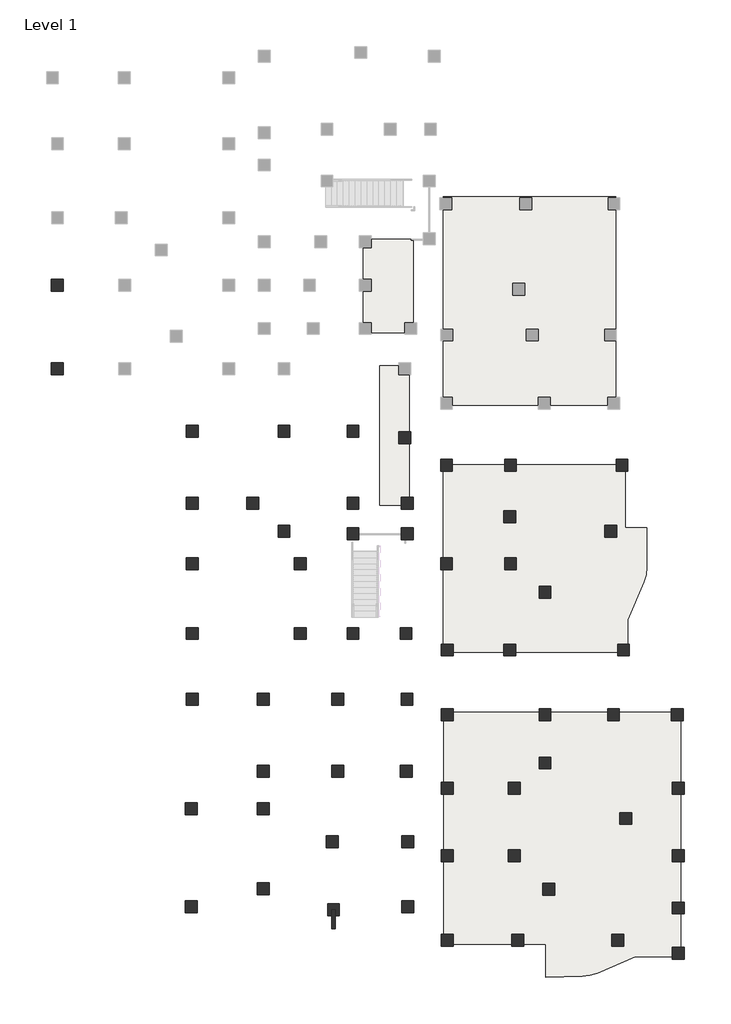
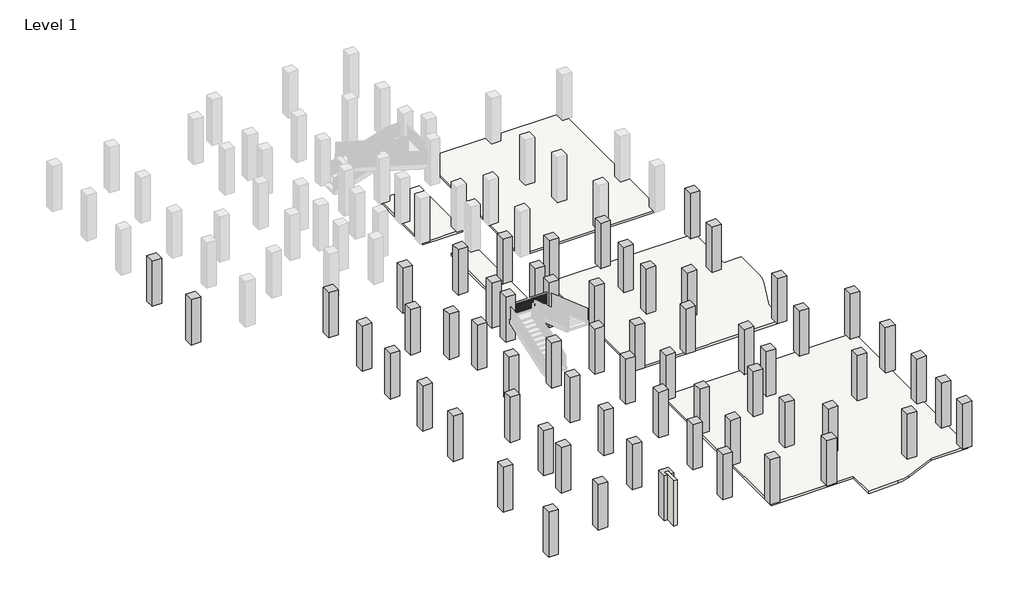
# One storey, part 1 of 6: 63 columns, 6 slabs, 1 wall.
"""IFC4 building model written with IfcOpenShell, lengths in millimetres."""

from ifc_helpers import new_model, si_unit, point, frame, frame_2d, origin, origin_with_axes, place, context, project, spatial, polyline, circle_curve, trimmed, segment, composite_curve, outline, extrude, faceted_brep, element, save

model = new_model("IFC4")

# Units and contexts
model_context = context("Model", 3, world=origin())
ifc_project = project(units=[si_unit("LENGTHUNIT", "METRE", prefix="MILLI")], contexts=[model_context])

# Site, building, storey
site = spatial("IfcSite", under=ifc_project)
building = spatial("IfcBuilding", under=site)
storey = spatial("IfcBuildingStorey", under=building, Name="Level 1", Elevation=0.0)

# Columns
placement = place(None, origin())
element("IfcColumn", 1, ObjectType="Rectangular Column : 24\" x 24\"", at=placement, inside=storey, context=model_context, shape_type="SweptSolid", body=[
    extrude(outline(polyline([(-4542.8891351, -24693.9416506), (-4542.8891351, -25303.5416506), (-4746.0891351, -25303.5416506), (-4746.0891351, -24998.7416506), (-4949.2891351, -24998.7416506), (-4949.2891351, -25303.5416506), (-5152.4891351, -25303.5416506), (-5152.4891351, -24693.9416506), (-4542.8891351, -24693.9416506)])), origin_with_axes(), (0.0, 0.0, 1.0), 3048.0),
])
element("IfcColumn", 2, ObjectType="Rectangular Column : 24\" x 24\"", at=placement, inside=storey, context=model_context, shape_type="SweptSolid", body=[
    extrude(outline(polyline([(-4321.237215, -17586.4072331), (-4321.237215, -18196.0072331), (-4930.837215, -18196.0072331), (-4930.837215, -17586.4072331), (-4321.237215, -17586.4072331)])), origin_with_axes(), (0.0, 0.0, 1.0), 3048.0),
])
element("IfcColumn", 3, ObjectType="Rectangular Column : 24\" x 24\"", at=placement, inside=storey, context=model_context, shape_type="SweptSolid", body=[
    extrude(outline(polyline([(-4600.0391351, -21207.7916506), (-4600.0391351, -21817.3916506), (-5209.6391351, -21817.3916506), (-5209.6391351, -21207.7916506), (-4600.0391351, -21207.7916506)])), origin_with_axes(), (0.0, 0.0, 1.0), 3048.0),
])
element("IfcColumn", 4, ObjectType="Rectangular Column : 24\" x 24\"", at=placement, inside=storey, context=model_context, shape_type="SweptSolid", body=[
    extrude(outline(polyline([(-11810.6574308, -13883.8238356), (-11810.6574308, -14493.4238356), (-12420.2574308, -14493.4238356), (-12420.2574308, -13883.8238356), (-11810.6574308, -13883.8238356)])), origin_with_axes(), (0.0, 0.0, 1.0), 3048.0),
])
element("IfcColumn", 5, ObjectType="Rectangular Column : 24\" x 24\"", at=placement, inside=storey, context=model_context, shape_type="SweptSolid", body=[
    extrude(outline(polyline([(-8149.0858024, -13883.8238356), (-8149.0858024, -14493.4238356), (-8758.6858024, -14493.4238356), (-8758.6858024, -13883.8238356), (-8149.0858024, -13883.8238356)])), origin_with_axes(), (0.0, 0.0, 1.0), 3048.0),
])
element("IfcColumn", 6, ObjectType="Rectangular Column : 24\" x 24\"", at=placement, inside=storey, context=model_context, shape_type="SweptSolid", body=[
    extrude(outline(polyline([(-4321.237215, -13883.8238356), (-4321.237215, -14493.4238356), (-4930.837215, -14493.4238356), (-4930.837215, -13883.8238356), (-4321.237215, -13883.8238356)])), origin_with_axes(), (0.0, 0.0, 1.0), 3048.0),
])
element("IfcColumn", 7, ObjectType="Rectangular Column : 24\" x 24\"", at=placement, inside=storey, context=model_context, shape_type="SweptSolid", body=[
    extrude(outline(polyline([(-766.6425319, -13883.8238356), (-766.6425319, -14493.4238356), (-1376.2425319, -14493.4238356), (-1376.2425319, -13883.8238356), (-766.6425319, -13883.8238356)])), origin_with_axes(), (0.0, 0.0, 1.0), 3048.0),
])
element("IfcColumn", 8, ObjectType="Rectangular Column : 24\" x 24\"", at=placement, inside=storey, context=model_context, shape_type="SweptSolid", body=[
    extrude(outline(polyline([(-794.2108128, -17586.4072331), (-794.2108128, -18196.0072331), (-1403.8108128, -18196.0072331), (-1403.8108128, -17586.4072331), (-794.2108128, -17586.4072331)])), origin_with_axes(), (0.0, 0.0, 1.0), 3048.0),
])
element("IfcColumn", 9, ObjectType="Rectangular Column : 24\" x 24\"", at=placement, inside=storey, context=model_context, shape_type="SweptSolid", body=[
    extrude(outline(polyline([(-732.8891351, -21207.7916506), (-732.8891351, -21817.3916506), (-1342.4891351, -21817.3916506), (-1342.4891351, -21207.7916506), (-732.8891351, -21207.7916506)])), origin_with_axes(), (0.0, 0.0, 1.0), 3048.0),
])
element("IfcColumn", 10, ObjectType="Rectangular Column : 24\" x 24\"", at=placement, inside=storey, context=model_context, shape_type="SweptSolid", body=[
    extrude(outline(polyline([(-732.8891351, -24541.5416506), (-732.8891351, -25151.1416506), (-1342.4891351, -25151.1416506), (-1342.4891351, -24541.5416506), (-732.8891351, -24541.5416506)])), origin_with_axes(), (0.0, 0.0, 1.0), 3048.0),
])
element("IfcColumn", 11, ObjectType="Rectangular Column : 24\" x 24\"", at=placement, inside=storey, context=model_context, shape_type="SweptSolid", body=[
    extrude(outline(polyline([(-11858.0891351, -24541.5416506), (-11858.0891351, -25151.1416506), (-12467.6891351, -25151.1416506), (-12467.6891351, -24541.5416506), (-11858.0891351, -24541.5416506)])), origin_with_axes(), (0.0, 0.0, 1.0), 3048.0),
])
element("IfcColumn", 12, ObjectType="Rectangular Column : 24\" x 24\"", at=placement, inside=storey, context=model_context, shape_type="SweptSolid", body=[
    extrude(outline(polyline([(-11858.0891351, -19512.3416506), (-11858.0891351, -20121.9416506), (-12467.6891351, -20121.9416506), (-12467.6891351, -19512.3416506), (-11858.0891351, -19512.3416506)])), origin_with_axes(), (0.0, 0.0, 1.0), 3048.0),
])
element("IfcColumn", 13, ObjectType="Rectangular Column : 24\" x 24\"", at=placement, inside=storey, context=model_context, shape_type="SweptSolid", body=[
    extrude(outline(polyline([(-8149.0858024, -17586.4072331), (-8149.0858024, -18196.0072331), (-8758.6858024, -18196.0072331), (-8758.6858024, -17586.4072331), (-8149.0858024, -17586.4072331)])), origin_with_axes(), (0.0, 0.0, 1.0), 3048.0),
])
element("IfcColumn", 14, ObjectType="Rectangular Column : 24\" x 24\"", at=placement, inside=storey, context=model_context, shape_type="SweptSolid", body=[
    extrude(outline(polyline([(-8149.0858024, -19512.3416506), (-8149.0858024, -20121.9416506), (-8758.6858024, -20121.9416506), (-8758.6858024, -19512.3416506), (-8149.0858024, -19512.3416506)])), origin_with_axes(), (0.0, 0.0, 1.0), 3048.0),
])
element("IfcColumn", 15, ObjectType="Rectangular Column : 24\" x 24\"", at=placement, inside=storey, context=model_context, shape_type="SweptSolid", body=[
    extrude(outline(polyline([(-8149.0858024, -23627.1416506), (-8149.0858024, -24236.7416506), (-8758.6858024, -24236.7416506), (-8758.6858024, -23627.1416506), (-8149.0858024, -23627.1416506)])), origin_with_axes(), (0.0, 0.0, 1.0), 3048.0),
])
element("IfcColumn", 16, ObjectType="Rectangular Column : 24\" x 24\"", at=placement, inside=storey, context=model_context, shape_type="SweptSolid", body=[
    extrude(outline(polyline([(1308.8550323, -26276.0205306), (1308.8550323, -26885.6205306), (699.2550323, -26885.6205306), (699.2550323, -26276.0205306), (1308.8550323, -26276.0205306)])), origin_with_axes(), (0.0, 0.0, 1.0), 3048.0),
])
element("IfcColumn", 17, ObjectType="Rectangular Column : 24\" x 24\"", at=placement, inside=storey, context=model_context, shape_type="SweptSolid", body=[
    extrude(outline(polyline([(4934.0839763, -26276.0205306), (4934.0839763, -26885.6205306), (4324.4839763, -26885.6205306), (4324.4839763, -26276.0205306), (4934.0839763, -26276.0205306)])), origin_with_axes(), (0.0, 0.0, 1.0), 3048.0),
])
element("IfcColumn", 18, ObjectType="Rectangular Column : 24\" x 24\"", at=placement, inside=storey, context=model_context, shape_type="SweptSolid", body=[
    extrude(outline(polyline([(1308.8550323, -21920.2321416), (1308.8550323, -22529.8321416), (699.2550323, -22529.8321416), (699.2550323, -21920.2321416), (1308.8550323, -21920.2321416)])), origin_with_axes(), (0.0, 0.0, 1.0), 3048.0),
])
element("IfcColumn", 19, ObjectType="Rectangular Column : 24\" x 24\"", at=placement, inside=storey, context=model_context, shape_type="SweptSolid", body=[
    extrude(outline(polyline([(1308.8550323, -18453.3485113), (1308.8550323, -19062.9485113), (699.2550323, -19062.9485113), (699.2550323, -18453.3485113), (1308.8550323, -18453.3485113)])), origin_with_axes(), (0.0, 0.0, 1.0), 3048.0),
])
element("IfcColumn", 20, ObjectType="Rectangular Column : 24\" x 24\"", at=placement, inside=storey, context=model_context, shape_type="SweptSolid", body=[
    extrude(outline(polyline([(1308.8550323, -14677.1022473), (1308.8550323, -15286.7022473), (699.2550323, -15286.7022473), (699.2550323, -14677.1022473), (1308.8550323, -14677.1022473)])), origin_with_axes(), (0.0, 0.0, 1.0), 3048.0),
])
element("IfcColumn", 21, ObjectType="Rectangular Column : 24\" x 24\"", at=placement, inside=storey, context=model_context, shape_type="SweptSolid", body=[
    extrude(outline(polyline([(1308.8550323, -11343.8334596), (1308.8550323, -11953.4334596), (699.2550323, -11953.4334596), (699.2550323, -11343.8334596), (1308.8550323, -11343.8334596)])), origin_with_axes(), (0.0, 0.0, 1.0), 3048.0),
])
element("IfcColumn", 22, ObjectType="Rectangular Column : 24\" x 24\"", at=placement, inside=storey, context=model_context, shape_type="SweptSolid", body=[
    extrude(outline(polyline([(6333.7118156, -14677.1022473), (6333.7118156, -15286.7022473), (5724.1118156, -15286.7022473), (5724.1118156, -14677.1022473), (6333.7118156, -14677.1022473)])), origin_with_axes(), (0.0, 0.0, 1.0), 3048.0),
])
element("IfcColumn", 23, ObjectType="Rectangular Column : 24\" x 24\"", at=placement, inside=storey, context=model_context, shape_type="SweptSolid", body=[
    extrude(outline(polyline([(9855.6561951, -14677.1022473), (9855.6561951, -15286.7022473), (9246.0561951, -15286.7022473), (9246.0561951, -14677.1022473), (9855.6561951, -14677.1022473)])), origin_with_axes(), (0.0, 0.0, 1.0), 3048.0),
])
element("IfcColumn", 24, ObjectType="Rectangular Column : 24\" x 24\"", at=placement, inside=storey, context=model_context, shape_type="SweptSolid", body=[
    extrude(outline(polyline([(13126.0331188, -14677.1022473), (13126.0331188, -15286.7022473), (12516.4331188, -15286.7022473), (12516.4331188, -14677.1022473), (13126.0331188, -14677.1022473)])), origin_with_axes(), (0.0, 0.0, 1.0), 3048.0),
])
element("IfcColumn", 25, ObjectType="Rectangular Column : 24\" x 24\"", at=placement, inside=storey, context=model_context, shape_type="SweptSolid", body=[
    extrude(outline(polyline([(13188.9249828, -18453.3485113), (13188.9249828, -19062.9485113), (12579.3249828, -19062.9485113), (12579.3249828, -18453.3485113), (13188.9249828, -18453.3485113)])), origin_with_axes(), (0.0, 0.0, 1.0), 3048.0),
])
element("IfcColumn", 26, ObjectType="Rectangular Column : 24\" x 24\"", at=placement, inside=storey, context=model_context, shape_type="SweptSolid", body=[
    extrude(outline(polyline([(13188.9249828, -21920.2321416), (13188.9249828, -22529.8321416), (12579.3249828, -22529.8321416), (12579.3249828, -21920.2321416), (13188.9249828, -21920.2321416)])), origin_with_axes(), (0.0, 0.0, 1.0), 3048.0),
])
element("IfcColumn", 27, ObjectType="Rectangular Column : 24\" x 24\"", at=placement, inside=storey, context=model_context, shape_type="SweptSolid", body=[
    extrude(outline(polyline([(13188.9249828, -24614.0167464), (13188.9249828, -25223.6167464), (12579.3249828, -25223.6167464), (12579.3249828, -24614.0167464), (13188.9249828, -24614.0167464)])), origin_with_axes(), (0.0, 0.0, 1.0), 3048.0),
])
element("IfcColumn", 28, ObjectType="Rectangular Column : 24\" x 24\"", at=placement, inside=storey, context=model_context, shape_type="SweptSolid", body=[
    extrude(outline(polyline([(13188.9249828, -26941.0157114), (13188.9249828, -27550.6157114), (12579.3249828, -27550.6157114), (12579.3249828, -26941.0157114), (13188.9249828, -26941.0157114)])), origin_with_axes(), (0.0, 0.0, 1.0), 3048.0),
])
element("IfcColumn", 29, ObjectType="Rectangular Column : 24\" x 24\"", at=placement, inside=storey, context=model_context, shape_type="SweptSolid", body=[
    extrude(outline(polyline([(6531.1948888, -23643.0476028), (6531.1948888, -24252.6476028), (5921.5948888, -24252.6476028), (5921.5948888, -23643.0476028), (6531.1948888, -23643.0476028)])), origin_with_axes(), (0.0, 0.0, 1.0), 3048.0),
])
element("IfcColumn", 30, ObjectType="Rectangular Column : 24\" x 24\"", at=placement, inside=storey, context=model_context, shape_type="SweptSolid", body=[
    extrude(outline(polyline([(6330.6701053, -17153.3364275), (6330.6701053, -17762.9364275), (5721.0701053, -17762.9364275), (5721.0701053, -17153.3364275), (6330.6701053, -17153.3364275)])), origin_with_axes(), (0.0, 0.0, 1.0), 3048.0),
])
element("IfcColumn", 31, ObjectType="Rectangular Column : 24\" x 24\"", at=placement, inside=storey, context=model_context, shape_type="SweptSolid", body=[
    extrude(outline(polyline([(4744.701363, -18453.3485113), (4744.701363, -19062.9485113), (4135.101363, -19062.9485113), (4135.101363, -18453.3485113), (4744.701363, -18453.3485113)])), origin_with_axes(), (0.0, 0.0, 1.0), 3048.0),
])
element("IfcColumn", 32, ObjectType="Rectangular Column : 24\" x 24\"", at=placement, inside=storey, context=model_context, shape_type="SweptSolid", body=[
    extrude(outline(polyline([(4744.701363, -21920.2321416), (4744.701363, -22529.8321416), (4135.101363, -22529.8321416), (4135.101363, -21920.2321416), (4744.701363, -21920.2321416)])), origin_with_axes(), (0.0, 0.0, 1.0), 3048.0),
])
element("IfcColumn", 33, ObjectType="Rectangular Column : 24\" x 24\"", at=placement, inside=storey, context=model_context, shape_type="SweptSolid", body=[
    extrude(outline(polyline([(10492.7602331, -20012.0333502), (10492.7602331, -20621.6333502), (9883.1602331, -20621.6333502), (9883.1602331, -20012.0333502), (10492.7602331, -20012.0333502)])), origin_with_axes(), (0.0, 0.0, 1.0), 3048.0),
])
element("IfcColumn", 34, ObjectType="Rectangular Column : 24\" x 24\"", at=placement, inside=storey, context=model_context, shape_type="SweptSolid", body=[
    extrude(outline(polyline([(10072.0128709, -26276.0205306), (10072.0128709, -26885.6205306), (9462.4128709, -26885.6205306), (9462.4128709, -26276.0205306), (10072.0128709, -26276.0205306)])), origin_with_axes(), (0.0, 0.0, 1.0), 3048.0),
])
element("IfcColumn", 35, ObjectType="Rectangular Column : 24\" x 24\"", at=placement, inside=storey, context=model_context, shape_type="SweptSolid", body=[
    extrude(outline(polyline([(4518.3886201, -11343.8334596), (4518.3886201, -11953.4334596), (3908.7886201, -11953.4334596), (3908.7886201, -11343.8334596), (4518.3886201, -11343.8334596)])), origin_with_axes(), (0.0, 0.0, 1.0), 3048.0),
])
element("IfcColumn", 36, ObjectType="Rectangular Column : 24\" x 24\"", at=placement, inside=storey, context=model_context, shape_type="SweptSolid", body=[
    extrude(outline(polyline([(10367.3319646, -11343.8334596), (10367.3319646, -11953.4334596), (9757.7319646, -11953.4334596), (9757.7319646, -11343.8334596), (10367.3319646, -11343.8334596)])), origin_with_axes(), (0.0, 0.0, 1.0), 3048.0),
])
element("IfcColumn", 37, ObjectType="Rectangular Column : 24\" x 24\"", at=placement, inside=storey, context=model_context, shape_type="SweptSolid", body=[
    extrude(outline(polyline([(4560.3165294, -6918.1541185), (4560.3165294, -7527.7541185), (3950.7165294, -7527.7541185), (3950.7165294, -6918.1541185), (4560.3165294, -6918.1541185)])), origin_with_axes(), (0.0, 0.0, 1.0), 3048.0),
])
element("IfcColumn", 38, ObjectType="Rectangular Column : 24\" x 24\"", at=placement, inside=storey, context=model_context, shape_type="SweptSolid", body=[
    extrude(outline(polyline([(1268.975651, -6918.1541185), (1268.975651, -7527.7541185), (659.375651, -7527.7541185), (659.375651, -6918.1541185), (1268.975651, -6918.1541185)])), origin_with_axes(), (0.0, 0.0, 1.0), 3048.0),
])
element("IfcColumn", 39, ObjectType="Rectangular Column : 24\" x 24\"", at=placement, inside=storey, context=model_context, shape_type="SweptSolid", body=[
    extrude(outline(polyline([(1268.975651, -1847.7319933), (1268.975651, -2457.3319933), (659.375651, -2457.3319933), (659.375651, -1847.7319933), (1268.975651, -1847.7319933)])), origin_with_axes(), (0.0, 0.0, 1.0), 3048.0),
])
element("IfcColumn", 40, ObjectType="Rectangular Column : 24\" x 24\"", at=placement, inside=storey, context=model_context, shape_type="SweptSolid", body=[
    extrude(outline(polyline([(4560.3165294, -1847.7319933), (4560.3165294, -2457.3319933), (3950.7165294, -2457.3319933), (3950.7165294, -1847.7319933), (4560.3165294, -1847.7319933)])), origin_with_axes(), (0.0, 0.0, 1.0), 3048.0),
])
element("IfcColumn", 41, ObjectType="Rectangular Column : 24\" x 24\"", at=placement, inside=storey, context=model_context, shape_type="SweptSolid", body=[
    extrude(outline(polyline([(10293.0740996, -1847.7319933), (10293.0740996, -2457.3319933), (9683.4740996, -2457.3319933), (9683.4740996, -1847.7319933), (10293.0740996, -1847.7319933)])), origin_with_axes(), (0.0, 0.0, 1.0), 3048.0),
])
element("IfcColumn", 42, ObjectType="Rectangular Column : 24\" x 24\"", at=placement, inside=storey, context=model_context, shape_type="SweptSolid", body=[
    extrude(outline(polyline([(9706.0833697, -5246.6270738), (9706.0833697, -5856.2270738), (9096.4833697, -5856.2270738), (9096.4833697, -5246.6270738), (9706.0833697, -5246.6270738)])), origin_with_axes(), (0.0, 0.0, 1.0), 3048.0),
])
element("IfcColumn", 43, ObjectType="Rectangular Column : 24\" x 24\"", at=placement, inside=storey, context=model_context, shape_type="SweptSolid", body=[
    extrude(outline(polyline([(6333.7118156, -8377.9582897), (6333.7118156, -8987.5582897), (5724.1118156, -8987.5582897), (5724.1118156, -8377.9582897), (6333.7118156, -8377.9582897)])), origin_with_axes(), (0.0, 0.0, 1.0), 3048.0),
])
element("IfcColumn", 44, ObjectType="Rectangular Column : 24\" x 24\"", at=placement, inside=storey, context=model_context, shape_type="SweptSolid", body=[
    extrude(outline(polyline([(4518.3886201, -4496.4820882), (4518.3886201, -5106.0820882), (3908.7886201, -5106.0820882), (3908.7886201, -4496.4820882), (4518.3886201, -4496.4820882)])), origin_with_axes(), (0.0, 0.0, 1.0), 3048.0),
])
element("IfcColumn", 45, ObjectType="Rectangular Column : 24\" x 24\"", at=placement, inside=storey, context=model_context, shape_type="SweptSolid", body=[
    extrude(outline(polyline([(-3540.2090245, -3808.9159518), (-3540.2090245, -4418.5159518), (-4149.8090245, -4418.5159518), (-4149.8090245, -3808.9159518), (-3540.2090245, -3808.9159518)])), origin_with_axes(), (0.0, 0.0, 1.0), 3048.0),
])
element("IfcColumn", 46, ObjectType="Rectangular Column : 24\" x 24\"", at=placement, inside=storey, context=model_context, shape_type="SweptSolid", body=[
    extrude(outline(polyline([(-3540.2090245, -5366.5238251), (-3540.2090245, -5976.1238251), (-4149.8090245, -5976.1238251), (-4149.8090245, -5366.5238251), (-3540.2090245, -5366.5238251)])), origin_with_axes(), (0.0, 0.0, 1.0), 3048.0),
])
element("IfcColumn", 47, ObjectType="Rectangular Column : 24\" x 24\"", at=placement, inside=storey, context=model_context, shape_type="SweptSolid", body=[
    extrude(outline(polyline([(-742.0285088, -5366.5238251), (-742.0285088, -5976.1238251), (-1351.6285088, -5976.1238251), (-1351.6285088, -5366.5238251), (-742.0285088, -5366.5238251)])), origin_with_axes(), (0.0, 0.0, 1.0), 3048.0),
])
element("IfcColumn", 48, ObjectType="Rectangular Column : 24\" x 24\"", at=placement, inside=storey, context=model_context, shape_type="SweptSolid", body=[
    extrude(outline(polyline([(-811.1636894, -10494.4811097), (-811.1636894, -11104.0811097), (-1420.7636894, -11104.0811097), (-1420.7636894, -10494.4811097), (-811.1636894, -10494.4811097)])), origin_with_axes(), (0.0, 0.0, 1.0), 3048.0),
])
element("IfcColumn", 49, ObjectType="Rectangular Column : 24\" x 24\"", at=placement, inside=storey, context=model_context, shape_type="SweptSolid", body=[
    extrude(outline(polyline([(-3540.2090245, -10494.4811097), (-3540.2090245, -11104.0811097), (-4149.8090245, -11104.0811097), (-4149.8090245, -10494.4811097), (-3540.2090245, -10494.4811097)])), origin_with_axes(), (0.0, 0.0, 1.0), 3048.0),
])
element("IfcColumn", 50, ObjectType="Rectangular Column : 24\" x 24\"", at=placement, inside=storey, context=model_context, shape_type="SweptSolid", body=[
    extrude(outline(polyline([(-6255.1201851, -10494.4811097), (-6255.1201851, -11104.0811097), (-6864.7201851, -11104.0811097), (-6864.7201851, -10494.4811097), (-6255.1201851, -10494.4811097)])), origin_with_axes(), (0.0, 0.0, 1.0), 3048.0),
])
element("IfcColumn", 51, ObjectType="Rectangular Column : 24\" x 24\"", at=placement, inside=storey, context=model_context, shape_type="SweptSolid", body=[
    extrude(outline(polyline([(-11810.6574308, -10494.4811097), (-11810.6574308, -11104.0811097), (-12420.2574308, -11104.0811097), (-12420.2574308, -10494.4811097), (-11810.6574308, -10494.4811097)])), origin_with_axes(), (0.0, 0.0, 1.0), 3048.0),
])
element("IfcColumn", 52, ObjectType="Rectangular Column : 24\" x 24\"", at=placement, inside=storey, context=model_context, shape_type="SweptSolid", body=[
    extrude(outline(polyline([(-6255.1201851, -6918.1541185), (-6255.1201851, -7527.7541185), (-6864.7201851, -7527.7541185), (-6864.7201851, -6918.1541185), (-6255.1201851, -6918.1541185)])), origin_with_axes(), (0.0, 0.0, 1.0), 3048.0),
])
element("IfcColumn", 53, ObjectType="Rectangular Column : 24\" x 24\"", at=placement, inside=storey, context=model_context, shape_type="SweptSolid", body=[
    extrude(outline(polyline([(-11810.6574308, -6918.1541185), (-11810.6574308, -7527.7541185), (-12420.2574308, -7527.7541185), (-12420.2574308, -6918.1541185), (-11810.6574308, -6918.1541185)])), origin_with_axes(), (0.0, 0.0, 1.0), 3048.0),
])
element("IfcColumn", 54, ObjectType="Rectangular Column : 24\" x 24\"", at=placement, inside=storey, context=model_context, shape_type="SweptSolid", body=[
    extrude(outline(polyline([(-7086.8650855, -5246.6270738), (-7086.8650855, -5856.2270738), (-7696.4650855, -5856.2270738), (-7696.4650855, -5246.6270738), (-7086.8650855, -5246.6270738)])), origin_with_axes(), (0.0, 0.0, 1.0), 3048.0),
])
element("IfcColumn", 55, ObjectType="Rectangular Column : 24\" x 24\"", at=placement, inside=storey, context=model_context, shape_type="SweptSolid", body=[
    extrude(outline(polyline([(-8694.9052261, -3808.9159518), (-8694.9052261, -4418.5159518), (-9304.5052261, -4418.5159518), (-9304.5052261, -3808.9159518), (-8694.9052261, -3808.9159518)])), origin_with_axes(), (0.0, 0.0, 1.0), 3048.0),
])
element("IfcColumn", 56, ObjectType="Rectangular Column : 24\" x 24\"", at=placement, inside=storey, context=model_context, shape_type="SweptSolid", body=[
    extrude(outline(polyline([(-11810.6574308, -3808.9159518), (-11810.6574308, -4418.5159518), (-12420.2574308, -4418.5159518), (-12420.2574308, -3808.9159518), (-11810.6574308, -3808.9159518)])), origin_with_axes(), (0.0, 0.0, 1.0), 3048.0),
])
element("IfcColumn", 57, ObjectType="Rectangular Column : 24\" x 24\"", at=placement, inside=storey, context=model_context, shape_type="SweptSolid", body=[
    extrude(outline(polyline([(-11810.6574308, -106.2126672), (-11810.6574308, -715.8126672), (-12420.2574308, -715.8126672), (-12420.2574308, -106.2126672), (-11810.6574308, -106.2126672)])), origin_with_axes(), (0.0, 0.0, 1.0), 3048.0),
])
element("IfcColumn", 58, ObjectType="Rectangular Column : 24\" x 24\"", at=placement, inside=storey, context=model_context, shape_type="SweptSolid", body=[
    extrude(outline(polyline([(-7086.8650855, -106.2126672), (-7086.8650855, -715.8126672), (-7696.4650855, -715.8126672), (-7696.4650855, -106.2126672), (-7086.8650855, -106.2126672)])), origin_with_axes(), (0.0, 0.0, 1.0), 3048.0),
])
element("IfcColumn", 59, ObjectType="Rectangular Column : 24\" x 24\"", at=placement, inside=storey, context=model_context, shape_type="SweptSolid", body=[
    extrude(outline(polyline([(-3540.2090245, -106.2126672), (-3540.2090245, -715.8126672), (-4149.8090245, -715.8126672), (-4149.8090245, -106.2126672), (-3540.2090245, -106.2126672)])), origin_with_axes(), (0.0, 0.0, 1.0), 3048.0),
])
element("IfcColumn", 60, ObjectType="Rectangular Column : 24\" x 24\"", at=placement, inside=storey, context=model_context, shape_type="SweptSolid", body=[
    extrude(outline(polyline([(-742.0285088, -3808.9159518), (-742.0285088, -4418.5159518), (-1351.6285088, -4418.5159518), (-1351.6285088, -3808.9159518), (-742.0285088, -3808.9159518)])), origin_with_axes(), (0.0, 0.0, 1.0), 3048.0),
])
element("IfcColumn", 61, ObjectType="Rectangular Column : 24\" x 24\"", at=placement, inside=storey, context=model_context, shape_type="SweptSolid", body=[
    extrude(outline(polyline([(-881.5354844, -434.4941146), (-881.5354844, -1044.0941146), (-1491.1354844, -1044.0941146), (-1491.1354844, -434.4941146), (-881.5354844, -434.4941146)])), origin_with_axes(), (0.0, 0.0, 1.0), 3048.0),
])
element("IfcColumn", 62, ObjectType="Rectangular Column : 24\" x 24\"", at=placement, inside=storey, context=model_context, shape_type="SweptSolid", body=[
    extrude(outline(polyline([(-18746.2659238, 3108.0299865), (-18746.2659238, 2498.4299865), (-19355.8659238, 2498.4299865), (-19355.8659238, 3108.0299865), (-18746.2659238, 3108.0299865)])), origin_with_axes(), (0.0, 0.0, 1.0), 3048.0),
])
element("IfcColumn", 63, ObjectType="Rectangular Column : 24\" x 24\"", at=placement, inside=storey, context=model_context, shape_type="SweptSolid", body=[
    extrude(outline(polyline([(-18746.2659238, 7403.6904836), (-18746.2659238, 6794.0904836), (-19355.8659238, 6794.0904836), (-19355.8659238, 7403.6904836), (-18746.2659238, 7403.6904836)])), origin_with_axes(), (0.0, 0.0, 1.0), 3048.0),
])

# Slabs
element("IfcSlab", 64, ObjectType="Generic - 12\"", at=placement, inside=storey, context=model_context, shape_type="SweptSolid", body=[
    extrude(outline(composite_curve([segment(polyline([(13017.3380523, -27431.6042694), (10660.5280667, -27431.6042694), (8711.1928652, -28266.3478094)]), True, "CONTINUOUS"), segment(trimmed(circle_curve(frame_2d((7951.2985405, -26491.8042694)), 1930.4), [point((8711.1928652, -28266.3478094))], [point((7953.0959373, -28422.2034326))], False, "CARTESIAN"), True, "CONTINUOUS"), segment(polyline([(7953.0959373, -28422.2034326), (6070.4380523, -28487.9472947), (6070.4380523, -26783.9042694), (812.6380523, -26783.9042694), (812.6380523, -14845.9042694), (13017.3380523, -14845.9042694), (13017.3380523, -27431.6042694)]), True, "CONTINUOUS")], self_intersect=False)), frame((0.0, 0.0, -152.4), z_axis=(0.0, 0.0, 1.0), x_axis=(1.0, 0.0, 0.0)), (0.0, 0.0, 1.0), 152.4),
])
element("IfcSlab", 65, ObjectType="Generic - 12\"", at=placement, inside=storey, context=model_context, shape_type="SweptSolid", body=[
    extrude(outline(composite_curve([segment(polyline([(10274.1380523, -11759.8042694), (803.8108649, -11759.8042694), (803.8108649, -2133.2042694), (10159.8380523, -2133.2042694), (10159.8380523, -5352.6542694), (11264.7380523, -5352.6542694), (11264.7380523, -7397.5810633)]), True, "CONTINUOUS"), segment(trimmed(circle_curve(frame_2d((9334.3380523, -7397.5810633)), 1930.4), [point((11264.7380523, -7397.5810633))], [point((11108.8815923, -8157.475388))], False, "CARTESIAN"), True, "CONTINUOUS"), segment(polyline([(11108.8815923, -8157.475388), (10274.1380523, -10106.8105895), (10274.1380523, -11759.8042694)]), True, "CONTINUOUS")], self_intersect=False)), frame((0.0, 0.0, -152.4), z_axis=(0.0, 0.0, 1.0), x_axis=(1.0, 0.0, 0.0)), (0.0, 0.0, 1.0), 152.4),
])
element("IfcSlab", 66, ObjectType="Generic - 12\"", at=placement, inside=storey, context=model_context, shape_type="SweptSolid", body=[
    extrude(outline(polyline([(9677.2380523, 11646.2957306), (9677.2380523, 940.1957306), (793.5880523, 940.1957306), (793.5880523, 11646.2957306), (9677.2380523, 11646.2957306)])), frame((0.0, 0.0, -152.4), z_axis=(0.0, 0.0, 1.0), x_axis=(1.0, 0.0, 0.0)), (0.0, 0.0, 1.0), 152.4),
])
element("IfcSlab", 67, ObjectType="Generic - 12\"", at=placement, inside=storey, context=model_context, shape_type="SweptSolid", body=[
    extrude(outline(polyline([(-745.5891351, 9478.4949943), (-745.5891351, 4652.4949943), (-3310.9891351, 4652.4949943), (-3310.9891351, 9478.4949943), (-745.5891351, 9478.4949943)])), frame((0.0, 0.0, -152.4), z_axis=(0.0, 0.0, 1.0), x_axis=(1.0, 0.0, 0.0)), (0.0, 0.0, 1.0), 152.4),
])
element("IfcSlab", 68, ObjectType="Generic - 12\"", at=placement, inside=storey, context=model_context, shape_type="SweptSolid", body=[
    extrude(outline(polyline([(-961.4891351, 2953.9583494), (-961.4891351, -4202.4916506), (-2472.7891351, -4202.4916506), (-2472.7891351, 2953.9583494), (-961.4891351, 2953.9583494)])), frame((0.0, 0.0, -152.4), z_axis=(0.0, 0.0, 1.0), x_axis=(1.0, 0.0, 0.0)), (0.0, 0.0, 1.0), 152.4),
])
element("IfcSlab", 69, ObjectType="Generic - 12\"", at=placement, inside=storey, context=model_context, shape_type="SweptSolid", body=[
    extrude(outline(polyline([(-961.4891351, 2953.9583494), (-961.4891351, -4202.4916506), (-2472.7891351, -4202.4916506), (-2472.7891351, 2953.9583494), (-961.4891351, 2953.9583494)])), frame((0.0, 0.0, -152.4), z_axis=(0.0, 0.0, 1.0), x_axis=(1.0, 0.0, 0.0)), (0.0, 0.0, 1.0), 152.4),
])

# Wall
element("IfcWall", 70, ObjectType="9\" w", at=placement, inside=storey, context=model_context, shape_type="Brep", body=[
    faceted_brep([(-4746.0891351, -25989.3416506, 0.0), (-4746.0891351, -25303.5416506, 0.0), (-4746.0891351, -24998.7416506, 0.0), (-4746.0891351, -24998.7416506, 3048.0), (-4746.0891351, -25303.5416506, 3048.0), (-4746.0891351, -25989.3416506, 3048.0), (-4949.2891351, -25989.3416506, 0.0), (-4949.2891351, -25989.3416506, 3048.0), (-4949.2891351, -25303.5416506, 3048.0), (-4949.2891351, -24998.7416506, 3048.0), (-4949.2891351, -24998.7416506, 0.0), (-4949.2891351, -25303.5416506, 0.0)], [[[0, 1, 2, 3, 4, 5]], [[6, 7, 8, 9, 10, 11]], [[2, 1, 0, 6, 11, 10]], [[3, 2, 10, 9]], [[5, 4, 3, 9, 8, 7]], [[0, 5, 7, 6]]]),
])

save(model, "model.ifc")

# Revit data of these elements
# Type "Rectangular Column : 24\" x 24\""
#   Assembly Code = "B1010200"
#   Depth = 2' - 0"
#   Offset Base = 0' - 0"
#   Offset Top = 0' - 0"
#   Width = 2' - 0"
#   Material = none
# Type "Generic - 12\""
#   Assembly Code = "B1010"
#   Function = 0
#   Layers, outside or top first: 0' - 6" no material (function 1)
# Type "9\" w"
#   Assembly Code = "B2010"
#   Layers, outside or top first: 0' - 8" no material (function 1)
# Element 1 (IfcColumn, "Rectangular Column : 24\" x 24\"")
#   Phase Created = New Construction
#   Materials on its faces: "Cherry", "Default Wall"
# Elements 2, 4, 5, 6, 13, 15, 22, 38, 40, 41, 45, 46, 49, 50, 52, 53, 55, 57, 59, 61, 63 (IfcColumn, "Rectangular Column : 24\" x 24\"")
#   Phase Created = New Construction
#   Materials on its faces: "Wood - Stained", "Cherry"
# Elements 3, 10, 11, 12, 14, 17, 21, 23, 24, 25, 26, 30, 33, 35, 36, 37, 39, 42, 43, 58, 60, 62 (IfcColumn, "Rectangular Column : 24\" x 24\"")
#   Phase Created = New Construction
#   Materials on its faces: "Cherry", "Wood - Stained"
# Elements 7, 8, 9, 18, 19, 20, 29, 31, 32, 47, 48, 51, 56 (IfcColumn, "Rectangular Column : 24\" x 24\"")
#   Phase Created = New Construction
#   Materials on its faces: "Wood - Stained"
# Elements 16, 27, 28, 34, 44, 54 (IfcColumn, "Rectangular Column : 24\" x 24\"")
#   Phase Created = New Construction
#   Materials on its faces: "Cherry"
# Elements 64, 65, 66, 67, 68, 69 (IfcSlab, "Generic - 12\"")
#   Height Offset From Level = 0' - 0"
#   Phase Created = New Construction
#   Materials on its faces: "Default Floor"
# Element 70 (IfcWall, "9\" w")
#   Top Offset = 0' - 0"
#   Base Offset = 0' - 0"
#   wall height = 10' - 0"
#   Phase Created = New Construction
#   Base Constraint = Level 1
#   Top Constraint = Level 2
#   Materials on its faces: "Cherry", "Default Wall"
# Materials
#   "Cherry": class "Wood", colour RGB 226 177 128, transparency 0, Description = "Prunus Serotina", Cost = 0
#   "Default Wall": colour RGB 128 128 128, transparency 0, Cost = 0
#   "Wood - Stained": class "Wood", colour RGB 224 178 126, transparency 0, Cost = 0
#   "Default Floor": colour RGB 128 128 128, transparency 0, Cost = 0
